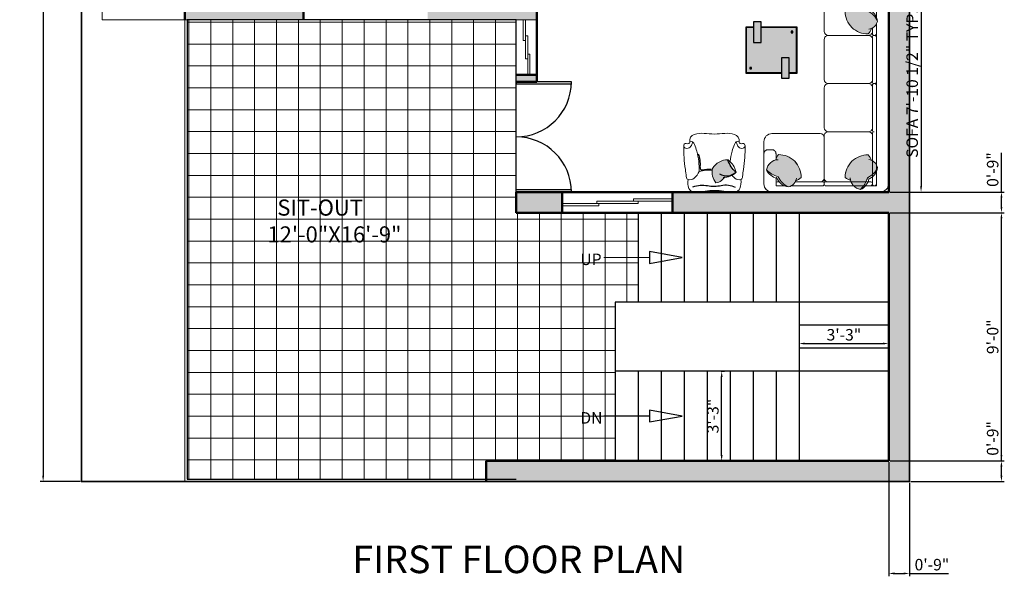
# Model space of a CAD drawing. Units: inches. Extents: x 1734 to 4011, y 1071 to 1891.
# Tile 24 of 27: x 3583 to 4011, y 1071 to 1313. Entities that reach past the tile are written whole.
import ezdxf

# ---------------------------------------------------------------- set-up
doc = ezdxf.new("R2010")
doc.units = ezdxf.units.IN
for name, color, linetype, lineweight in [('A-ANNO-DIMS', 2, 'Continuous', 18), ('A-ANNO-TEXT', 7, 'Continuous', 25), ('A-AREA-IDEN', 3, 'Continuous', 18), ('A-DOOR', 3, 'Continuous', 25), ('A-FLOR-OTLN', 7, 'Continuous', 25), ('A-FLOR-PATT', 252, 'Continuous', 13), ('A-FLOR-STRS', 2, 'Continuous', 25), ('A-FURN', 8, 'Continuous', 18), ('A-FURN-PATT', 252, 'Continuous', 13), ('A-GLAZ', 4, 'Continuous', 18), ('A-WALL', 7, 'Continuous', 50), ('A-WALL-PATT', 8, 'Continuous', 13), ('C-PROP', 1, 'Continuous', 35)]:
    doc.layers.add(name, color=color, linetype=linetype, lineweight=lineweight)
doc.layers.add('IFF-FURN-DETAIL', color=250, linetype='Continuous')
doc.layers.add('MOBIL', color=7, linetype='Continuous')
doc.styles.get("Standard").update_dxf_attribs({"font": 'arial.ttf'})
doc.dimstyles.new('ISO-25', dxfattribs={"dimtxt": 5, "dimasz": 2.5, "dimexe": 1.25, "dimexo": 0.625, "dimtad": 1, "dimdec": 1, "dimlunit": 3, "dimtxsty": 'Standard', "dimcen": 2.5, "dimclrt": 1, "dimadec": 0, "dimazin": 0, "dimtfac": 1, "dimtdec": 1, "dimtmove": 0, "dimatfit": 3, "dimfxl": 1, "dimarcsym": 0})

# ---------------------------------------------------------------- blocks, each defined once
blk = doc.blocks.new('*D59')
at = {"layer": 'A-ANNO-DIMS', "color": 0, "lineweight": -2, "transparency": 16777216}
for p, q in [((3609.2, 1831.82), (3591.89, 1831.82)), ((3593.14, 1829.32), (3593.14, 1114.32)), ((3609.2, 1111.82), (3591.89, 1111.82))]:
    blk.add_line(p, q, dxfattribs=at)
at = {"layer": 'A-ANNO-DIMS', "color": 0, "transparency": 16777216}
for points in [[(3592.73, 1829.32), (3593.56, 1829.32), (3593.14, 1831.82)], [(3592.73, 1114.32), (3593.56, 1114.32), (3593.14, 1111.82)]]:
    blk.add_solid(points, dxfattribs=at)
at = {"layer": 'Defpoints', "color": 0, "transparency": 16777216}
for p in [(3609.83, 1831.82), (3593.14, 1111.82), (3609.83, 1111.82)]:
    blk.add_point(p, dxfattribs=at)
at = {"layer": 'A-ANNO-DIMS', "color": 0, "transparency": 16777216, "insert": (3587.92, 1471.82), "char_height": 5, "attachment_point": 5, "rotation": 90}
blk.add_mtext("{\\H1.8x;60'}", dxfattribs=at)
blk = doc.blocks.new('*D60')
at = {"layer": 'A-ANNO-DIMS', "color": 0, "lineweight": -2, "transparency": 16777216}
for p, q in [((3888.02, 1159.82), (3889.43, 1159.82)), ((3888.18, 1123.32), (3888.18, 1157.32)), ((3888.02, 1120.82), (3889.43, 1120.82))]:
    blk.add_line(p, q, dxfattribs=at)
at = {"layer": 'A-ANNO-DIMS', "color": 0, "transparency": 16777216}
for points in [[(3887.76, 1157.32), (3888.59, 1157.32), (3888.18, 1159.82)], [(3887.76, 1123.32), (3888.59, 1123.32), (3888.18, 1120.82)]]:
    blk.add_solid(points, dxfattribs=at)
at = {"layer": 'Defpoints', "color": 0, "transparency": 16777216}
for p in [(3887.4, 1159.82), (3888.18, 1159.82), (3887.4, 1120.82)]:
    blk.add_point(p, dxfattribs=at)
at = {"layer": 'A-ANNO-DIMS', "color": 0, "transparency": 16777216, "insert": (3885, 1140.32), "char_height": 5, "attachment_point": 5, "rotation": 90}
blk.add_mtext('3\'-3"', dxfattribs=at)
blk = doc.blocks.new('*D61')
at = {"layer": 'A-ANNO-DIMS', "color": 0, "lineweight": -2, "transparency": 16777216}
for p, q in [((3921.83, 1174.19), (3921.83, 1170.62)), ((3960.83, 1174.19), (3960.83, 1170.62)), ((3924.33, 1171.87), (3958.33, 1171.87))]:
    blk.add_line(p, q, dxfattribs=at)
at = {"layer": 'A-ANNO-DIMS', "color": 0, "transparency": 16777216}
for points in [[(3924.33, 1172.28), (3924.33, 1171.45), (3921.83, 1171.87)], [(3958.33, 1172.28), (3958.33, 1171.45), (3960.83, 1171.87)]]:
    blk.add_solid(points, dxfattribs=at)
at = {"layer": 'Defpoints', "color": 0, "transparency": 16777216}
for p in [(3921.83, 1174.82), (3960.83, 1174.82), (3960.83, 1171.87)]:
    blk.add_point(p, dxfattribs=at)
at = {"layer": 'A-ANNO-DIMS', "color": 0, "transparency": 16777216, "insert": (3941.33, 1175.04), "char_height": 5, "attachment_point": 5}
blk.add_mtext('3\'-3"', dxfattribs=at)
blk = doc.blocks.new('Mesa de centro Cantria feeling')
at = {"layer": 'MOBIL', "ltscale": 0.2}
h = blk.add_hatch(color=256, dxfattribs=at)
h.set_gradient(color1=(74, 55, 38), color2=(104, 77, 54), one_color=1, tint=0.31, name='CYLINDER')
h.paths.add_polyline_path([(-0.85, -0.3), (-0.7, -0.3), (-0.7, 0.1), (-0.85, 0.1)])
h = blk.add_hatch(color=256, dxfattribs=at)
h.set_gradient(color1=(221, 221, 223), one_color=1, tint=1)
h.paths.add_polyline_path([(-0.15, -0.6), (-0.15, -0.89), (-0.01, -0.89), (-0.01, -0.01), (-0.7, -0.01), (-0.7, -0.3), (-0.85, -0.3), (-0.85, -0.01), (-0.99, -0.01), (-0.99, -0.89), (-0.3, -0.89), (-0.3, -0.6)])
h.paths.add_polyline_path([(-0.112, -0.112), (-0.112, -0.082), (-0.082, -0.082), (-0.082, -0.112)], flags=16)
h.paths.add_polyline_path([(-0.888, -0.788), (-0.888, -0.818), (-0.918, -0.818), (-0.918, -0.788)], flags=16)
h = blk.add_hatch(color=256, dxfattribs=at)
h.set_gradient(color1=(74, 55, 38), color2=(104, 77, 54), one_color=1, tint=0.31, name='CYLINDER')
h.paths.add_polyline_path([(-0.15, -0.6), (-0.3, -0.6), (-0.3, -1), (-0.15, -1)])
for points in [[(-0.85, 0), (-1, 0), (-1, -0.9), (-0.3, -0.9)], [(-0.15, -0.9), (0, -0.9), (0, 0), (-0.7, 0)], [(-0.85, -0.01), (-0.99, -0.01), (-0.99, -0.89), (-0.3, -0.89)], [(-0.15, -0.89), (-0.01, -0.89), (-0.01, -0.01), (-0.7, -0.01)]]:
    blk.add_lwpolyline(points, dxfattribs=at)
for points in [[(-0.85, -0.3), (-0.7, -0.3), (-0.7, 0.1), (-0.85, 0.1)], [(-0.082, -0.082), (-0.112, -0.082), (-0.112, -0.112), (-0.082, -0.112)], [(-0.15, -0.6), (-0.3, -0.6), (-0.3, -1), (-0.15, -1)], [(-0.918, -0.818), (-0.888, -0.818), (-0.888, -0.788), (-0.918, -0.788)]]:
    blk.add_lwpolyline(points, close=True, dxfattribs=at)
blk = doc.blocks.new("MD D 4'")
for p, q in [((0, 24), (0, 0)), ((1, 24), (1, 0)), ((47, 24), (47, 0)), ((48, 24), (48, 0)), ((0, 0), (1, 0)), ((48, 0), (47, 0))]:
    blk.add_line(p, q)
for centre, start, end in [((0, 0), 0, 90), ((48, 0), 90, 180)]:
    blk.add_arc(centre, 24, start, end)
blk = doc.blocks.new('SOFA 1')
at = {"transparency": 33554687}
h = blk.add_hatch(color=256, dxfattribs=at)
h.dxf.hatch_style = 1
h.paths.add_polyline_path([(3723.52, 1308.63, 0.147724), (3717.76, 1305.24, 0.310469), (3722.42, 1300.4), (3722.42, 1300.25, 0.156703), (3723.62, 1297.8, 0.425821), (3734.69, 1309.08, 0.121928), (3732.05, 1310.63, 0.233216), (3728.6, 1313.59, 0.213835)])
h = blk.add_hatch(color=256, dxfattribs=at)
h.dxf.hatch_style = 1
h.paths.add_polyline_path([(3769.65, 1307.6, 0.084911), (3767.15, 1309.12, 0.046133), (3766.46, 1311.13), (3759.18, 1311.13, 0.039409), (3758.92, 1310.24, 0.165523), (3756.31, 1309.02, 0.42585), (3767.59, 1297.95, 0.121928), (3769.15, 1300.58, 0.027403), (3769.65, 1300.83)])
h.paths.add_polyline_path([(3765.34, 1313.08), (3760.4, 1313.08, 0.097704), (3759.18, 1311.13), (3766.46, 1311.13, 0.04873)])
h.paths.add_polyline_path([(3763.76, 1314.88, 0.16488), (3760.4, 1313.08), (3765.34, 1313.08, 0.051917)])
h.paths.add_polyline_path([(3771.6, 1305.17, 0.090388), (3769.65, 1307.6), (3769.65, 1300.83, 0.136035), (3771.6, 1302.77)])
h = blk.add_hatch(color=256, dxfattribs=at)
h.dxf.hatch_style = 1
h.paths.add_polyline_path([(3769.16, 1235.96, 0.122267), (3767.6, 1238.61, 0.425972), (3756.32, 1227.54, 0.165563), (3758.93, 1226.32, 0.309481), (3763.76, 1221.69, 0.002677), (3763.83, 1221.72, 0.146094), (3767.16, 1227.43, 0.212433), (3772.1, 1232.48, 0.235342)])
h = blk.add_hatch(color=256, dxfattribs=at)
h.dxf.hatch_style = 1
h.paths.add_polyline_path([(3769.16, 1225.36, 0.122267), (3767.6, 1228.01, 0.425972), (3756.32, 1216.94, 0.165563), (3758.93, 1215.72, 0.309481), (3763.76, 1211.09, 0.002677), (3763.83, 1211.12, 0.146094), (3767.16, 1216.83, 0.212433), (3772.1, 1221.88, 0.235342)])
for p, q in [((3720.45, 1316.13), (3773.58, 1316.13)), ((3777.51, 1312.19), (3777.51, 1213.72))]:
    blk.add_line(p, q, dxfattribs=at)
for points in [[(3716.51, 1312.2), (3716.51, 1291.44)], [(3722.42, 1313.08), (3722.42, 1309.23), (3722.42, 1313.08), (3726.57, 1313.08)], [(3729.85, 1313.08), (3745.25, 1313.08)], [(3746.01, 1312.3), (3746.01, 1288.55)], [(3768.11, 1313.08), (3746.78, 1313.08)], [(3771.6, 1313.08), (3767.75, 1313.08), (3771.6, 1313.08), (3771.6, 1308.93)], [(3769.66, 1287.39), (3769.65, 1312.3)], [(3771.6, 1313.08), (3771.61, 1233.74)], [(3723.21, 1311.13), (3723.93, 1311.13)], [(3731.82, 1311.13), (3745.25, 1311.13)], [(3746.01, 1310.97), (3746.01, 1311.36)], [(3746.01, 1288.54), (3746.01, 1308.23)], [(3768.87, 1311.13), (3746.78, 1311.13)], [(3769.65, 1309.43), (3769.65, 1308.71)], [(3722.42, 1300.39), (3722.42, 1297.33)], [(3720.45, 1295.38), (3718.48, 1295.38)], [(3720.45, 1287.5), (3744.09, 1287.5)], [(3746.02, 1284.63), (3746.02, 1264.94)], [(3747.99, 1286.6), (3767.69, 1286.6)], [(3769.66, 1263.75), (3769.66, 1285.81)], [(3769.66, 1277.18), (3769.66, 1263.75)], [(3746.02, 1260.99), (3746.02, 1241.3)], [(3747.99, 1262.97), (3767.69, 1262.97)], [(3769.66, 1240.12), (3769.66, 1262.18)], [(3770.43, 1262.97), (3770.82, 1262.97)], [(3746.02, 1237.36), (3746.02, 1213.74)], [(3747.99, 1239.33), (3767.69, 1239.33)], [(3769.66, 1235.71), (3769.66, 1238.54)], [(3770.43, 1239.33), (3770.82, 1239.33)], [(3771.61, 1223.14), (3771.61, 1230.47)], [(3769.66, 1225.11), (3769.66, 1227.82)], [(3755.86, 1215.72), (3758.92, 1215.72)], [(3767.76, 1215.72), (3771.61, 1215.72), (3771.61, 1219.84), (3771.61, 1215.72)], [(3769.66, 1216.5), (3769.66, 1217.22)], [(3753.91, 1211.77), (3753.91, 1213.74)], [(3749.97, 1209.8), (3773.58, 1209.8)]]:
    blk.add_lwpolyline(points, close=True, dxfattribs=at)
for points in [[(3717.76, 1305.24, -0.147724), (3723.52, 1308.63, -0.213355), (3728.59, 1313.59, 0.213355), (3723.52, 1308.63, 0.147724), (3717.76, 1305.24, -0.249545), (3722.86, 1309.34, 0.249545), (3717.75, 1305.25, 0.356779), (3723.4, 1300.28, -0.356779), (3717.76, 1305.24)], [(3728.58, 1313.6, -0.306333), (3732.42, 1309.31, 0.306333), (3728.58, 1313.6, 0.306674), (3722.72, 1308.89, -0.306674), (3728.58, 1313.6)], [(3763.76, 1314.88, -0.147724), (3767.15, 1309.12, -0.213355), (3772.1, 1304.05, 0.213355), (3767.15, 1309.12, 0.147724), (3763.76, 1314.88, -0.249545), (3767.86, 1309.77, 0.249545), (3763.77, 1314.89, 0.356779), (3758.8, 1309.23, -0.356779), (3763.76, 1314.88)], [(3734.69, 1309.08, -0.425972), (3723.62, 1297.8, -0.165552), (3722.4, 1300.4, 0.165552), (3723.62, 1297.79, 0.425972), (3734.69, 1309.07, 0.121514), (3732.07, 1310.63, -0.121514), (3734.69, 1309.08)], [(3767.6, 1297.95, -0.425972), (3756.31, 1309.01, -0.165552), (3758.92, 1310.24, 0.165552), (3756.31, 1309.02, 0.425972), (3767.59, 1297.95, 0.121514), (3769.14, 1300.57, -0.121514), (3767.6, 1297.95)], [(3772.11, 1304.06, -0.306333), (3767.83, 1300.22, 0.306333), (3772.11, 1304.06, 0.306674), (3767.4, 1309.91, -0.306674), (3772.11, 1304.06)], [(3770.44, 1286.63, -0.414214), (3769.66, 1287.4, 0.414214), (3770.44, 1286.63, 0.414214), (3769.66, 1285.83, -0.414214), (3770.44, 1286.63)], [(3748.01, 1262.99, -0.414214), (3746.05, 1264.95, 0.414214), (3748.01, 1262.97, 0.414213), (3746.05, 1261.01, -0.414213), (3748.01, 1262.99)], [(3770.44, 1262.99, -0.414214), (3769.66, 1263.77, 0.414214), (3770.44, 1262.99, 0.414214), (3769.66, 1262.19, -0.414214), (3770.44, 1262.99)], [(3770.83, 1262.97, -0.414214), (3771.61, 1262.19, 0.414214), (3770.83, 1262.99, 0.414214), (3771.61, 1263.77, -0.414214), (3770.83, 1262.97)], [(3748.01, 1239.35, -0.414214), (3746.05, 1241.31, 0.414214), (3748.01, 1239.33, 0.414213), (3746.05, 1237.37, -0.414213), (3748.01, 1239.35)], [(3767.7, 1239.33, -0.414214), (3769.66, 1237.37, 0.414214), (3767.7, 1239.35, 0.414214), (3769.66, 1241.31, -0.414214), (3767.7, 1239.33)], [(3770.44, 1239.35, -0.414214), (3769.66, 1240.13, 0.414214), (3770.44, 1239.33, 0.414214), (3769.66, 1238.55, -0.414214), (3770.44, 1239.35)], [(3770.83, 1239.33, -0.414214), (3771.61, 1238.55, 0.414214), (3770.83, 1239.35, 0.414214), (3771.61, 1240.13, -0.414214), (3770.83, 1239.33)], [(3756.32, 1227.54, -0.425972), (3767.6, 1238.61, -0.121514), (3769.16, 1235.98, 0.121514), (3767.6, 1238.61, 0.425972), (3756.32, 1227.54, 0.165552), (3758.93, 1226.32, -0.165552), (3756.32, 1227.54)], [(3772.1, 1232.5, -0.306674), (3767.41, 1226.64, 0.306674), (3772.1, 1232.5, 0.306333), (3767.84, 1236.34, -0.306333), (3772.1, 1232.5)], [(3763.78, 1221.67, 0.249545), (3767.87, 1226.78, -0.249545), (3763.76, 1221.69, -0.356779), (3758.81, 1227.32, 0.356779), (3763.77, 1221.68, 0.147724), (3767.16, 1227.43, 0.213355), (3772.11, 1232.51, -0.213355), (3767.16, 1227.43, -0.147724), (3763.78, 1221.67)], [(3756.32, 1216.94, -0.200233), (3759.49, 1224.76, 0.200233), (3756.32, 1216.94, 0.165552), (3758.93, 1215.72, -0.165552), (3756.32, 1216.94)], [(3772.1, 1221.9, -0.306674), (3767.41, 1216.04, 0.306674), (3772.1, 1221.9, -0.213355), (3767.16, 1216.83, -0.147724), (3763.77, 1211.08, 0.147724), (3767.15, 1216.83, 0.213355), (3772.1, 1221.9)], [(3763.76, 1211.09, -0.356779), (3758.81, 1216.72, 0.356779), (3763.76, 1211.09, 0.249545), (3767.87, 1216.18, -0.249545), (3763.76, 1211.09)]]:
    blk.add_lwpolyline(points, format="xyb", dxfattribs=at)
for points in [[(3722.42, 1311.91, 0.414214), (3723.2, 1311.13, -0.414214)], [(3770.43, 1313.08, 0.414214), (3769.65, 1312.3, -0.414214)], [(3771.6, 1312.3, 0.414214), (3770.82, 1313.08, -0.414214)], [(3716.51, 1297.34, 0.414214), (3718.47, 1295.38, -0.414214)], [(3720.44, 1295.38, 0.414214), (3722.4, 1297.34, -0.414214)], [(3716.51, 1291.45, 0.414212), (3720.44, 1287.52, -0.414212)], [(3746.03, 1288.56, 0.414214), (3747.99, 1286.6, 0.414213), (3746.03, 1284.64, -0.414213), (3747.99, 1286.6, -0.414214)], [(3769.66, 1284.64, 0.414214), (3767.7, 1286.6, 0.414214), (3769.66, 1288.56, -0.414214), (3767.7, 1286.6, -0.414214)], [(3769.66, 1261.01, 0.414214), (3767.7, 1262.97, 0.414214), (3769.66, 1264.93, -0.414214), (3767.7, 1262.97, -0.414214)], [(3772.13, 1221.9, 0.306333), (3767.84, 1225.74, -0.306333)], [(3769.16, 1225.36, 0.071861), (3768.39, 1227.01, -0.071861)], [(3755.87, 1215.72, 0.414214), (3753.91, 1213.76, -0.414214)], [(3769.66, 1216.52, 0.414214), (3770.44, 1215.74, -0.414214)], [(3770.83, 1215.74, 0.414214), (3771.61, 1216.52, -0.414214)], [(3746.05, 1213.76, 0.414212), (3749.98, 1209.82, -0.414212)], [(3755.87, 1209.8, -0.414214), (3753.91, 1211.76, 0.414214)]]:
    blk.add_lwpolyline(points, format="xyb", close=True, dxfattribs=at)
for centre, radius, start, end in [((3720.44, 1312.2), 3.93, 90.0002, 179.9998), ((3720.44, 1312.19), 3.94, 89.9158, 179.9154), ((3745.22, 1312.29), 0.789, 0.8425, 90.8425), ((3745.24, 1311.91), 0.777, 270, 0), ((3745.24, 1311.91), 0.777, 270, 0), ((3746.8, 1312.29), 0.789, 89.1575, 179.1575), ((3746.79, 1311.91), 0.777, 180, 270), ((3746.79, 1311.91), 0.777, 180, 270), ((3768.87, 1312.3), 0.777, 360, 90), ((3768.87, 1311.91), 0.777, 270, 0), ((3773.58, 1312.2), 3.93, 0.0002, 89.9998), ((3773.57, 1312.19), 3.94, 359.9158, 89.9154), ((3744.09, 1309.21), 1.92, 358.766, 90.5111), ((3747.93, 1309.21), 1.92, 89.4889, 181.234), ((3744.08, 1289.48), 1.96, 270, 360), ((3744.08, 1289.48), 1.96, 270, 360), ((3773.58, 1213.73), 3.93, 270.0002, 359.9998), ((3773.59, 1213.73), 3.93, 269.9156, 359.9152)]:
    blk.add_arc(centre, radius, start, end, dxfattribs=at)
blk = doc.blocks.new('PILLOW-1')
at = {"color": 0}
blk.add_lwpolyline([(198, -165, -0.232884), (126, -346, -0.184752), (-44, -234, -0.286563), (75, -22, -0.237978), (273, -68, -0.243587), (179, -195, 4.263709)], format="xyb", dxfattribs=at)
at = {"layer": 'IFF-FURN-DETAIL'}
blk.add_lwpolyline([(148, -118, -0.343333), (126, -342, 0.126408), (-40, -233, -5.969376)], format="xyb", dxfattribs=at)
blk = doc.blocks.new('CLNG90')
for points in [[(689, 370, 0.157831), (677, 385, 0.121013), (646, 395, -0.017334), (547, 407, 0.041496), (215, 431, 0.153531), (191, 423, 0.382906), (185, 395, -0.284047), (184, 361, 0.011997), (177, 351, -0.370479), (160, 345, 0.380647), (56, 282, 0.117468), (41, 146, -0.027775), (50, 0, -8.773898)], [(160, 345, 0.22481), (160, 306, 0.055398), (209, 322, 0.180116), (249, 368, 0.194833), (248, 405, 0.242377), (215, 431, 1.52074)], [(160, 345, 0.22481), (160, 306, 0.055398), (209, 322, 0.180116), (249, 368, 0.194833), (248, 405, 0.242377), (215, 431, 1.52074)], [(689, 370, -0.235486), (671, 286, -0.134038), (574, 215, -0.079303), (293, 248, -0.027048), (199, 280, -0.106276), (160, 306, -1.699)], [(689, 370, -0.235486), (671, 286, -0.134038), (574, 215, -0.079303), (293, 248, -0.027048), (199, 280, -0.106276), (160, 306, -1.699)], [(689, 370, -0.146607), (814, 357, -0.305296), (862, 286, -0.042137), (852, 131, 0.040285), (843, 0, 3.952121)], [(574, 215, 0.061244), (556, 29, 3.376255)], [(574, 215, 0.061244), (556, 29, 3.376255)], [(689, -370, -0.157831), (677, -385, -0.121013), (646, -395, 0.017334), (547, -407, -0.041496), (215, -431, -0.153531), (191, -423, -0.382906), (185, -395, 0.284047), (184, -361, -0.011997), (177, -351, 0.370479), (160, -345, -0.380647), (56, -282, -0.117468), (41, -146, 0.027775), (50, 0, 8.773898)], [(689, -370, 0.146607), (814, -357, 0.305296), (862, -286, 0.042137), (852, -131, -0.040285), (843, 0, -3.952121)], [(437, -220, 0.041086), (293, -248, 0.027048), (199, -280, 0.106276), (160, -306, 1.699)], [(437, -220, 0.041086), (293, -248, 0.027048), (199, -280, 0.106276), (160, -306, 1.699)], [(689, -370, 0.235486), (671, -286, 0.060693), (632, -247, 0.001296)], [(689, -370, 0.235486), (671, -286, 0.060693), (632, -247, 0.001296)], [(160, -345, -0.22481), (160, -306, -0.055398), (209, -322, -0.180116), (249, -368, -0.194833), (248, -405, -0.242377), (215, -431, -1.52074)], [(160, -345, -0.22481), (160, -306, -0.055398), (209, -322, -0.180116), (249, -368, -0.194833), (248, -405, -0.242377), (215, -431, -1.52074)]]:
    blk.add_lwpolyline(points, format="xyb")
at = {"layer": 'IFF-FURN-DETAIL'}
for points in [[(791, 301, 0.124986), (774, 96, -0.091334), (771, -95, 0.164688), (797, -292, 1.068868)], [(791, 301, 0.124986), (774, 96, -0.091334), (771, -95, 0.164688), (797, -292, 1.068868)], [(328, 228, 0.109125), (508, 203, -0.16587), (546, 194, -0.314359), (555, 172, 0.072017), (544, 42, 4.351186)], [(328, 228, 0.109125), (508, 203, -0.16587), (546, 194, -0.314359), (555, 172, 0.072017), (544, 42, 4.351186)]]:
    blk.add_lwpolyline(points, format="xyb", dxfattribs=at)
at = {"xscale": 1.016, "yscale": 1.016, "zscale": 1.016}
blk.add_blockref('PILLOW-1', (458, 47), dxfattribs=at)
blk.add_blockref('PILLOW-1', (458, 47), dxfattribs=at)
blk = doc.blocks.new('*D85')
at = {"layer": 'A-ANNO-DIMS', "color": 0, "lineweight": -2, "transparency": 16777216}
for p, q in [((3961.35, 1332.21), (3976.13, 1332.21)), ((3974.88, 1329.71), (3974.88, 1240.32)), ((3961.35, 1237.82), (3976.13, 1237.82))]:
    blk.add_line(p, q, dxfattribs=at)
at = {"layer": 'A-ANNO-DIMS', "color": 0, "transparency": 16777216}
for points in [[(3974.47, 1329.71), (3975.3, 1329.71), (3974.88, 1332.21)], [(3974.47, 1240.32), (3975.3, 1240.32), (3974.88, 1237.82)]]:
    blk.add_solid(points, dxfattribs=at)
at = {"layer": 'Defpoints', "color": 0, "transparency": 16777216}
for p in [(3960.72, 1332.21), (3960.72, 1237.82), (3974.88, 1237.82)]:
    blk.add_point(p, dxfattribs=at)
at = {"layer": 'A-ANNO-DIMS', "color": 1, "transparency": 16777216, "insert": (3971.67, 1285.01), "char_height": 5, "attachment_point": 5, "rotation": 90}
blk.add_mtext('SOFA 7\'-10 1/2" TYP.', dxfattribs=at)
blk = doc.blocks.new('*D131')
at = {"layer": 'A-ANNO-DIMS', "color": 0, "lineweight": -2, "transparency": 16777216}
for p, q in [((4009.83, 1120.82), (4009.83, 1137.86)), ((3961.45, 1120.82), (4011.08, 1120.82)), ((4009.83, 1114.32), (4009.83, 1118.32)), ((3970.45, 1111.82), (4011.08, 1111.82))]:
    blk.add_line(p, q, dxfattribs=at)
at = {"layer": 'A-ANNO-DIMS', "color": 0, "transparency": 16777216}
for points in [[(4009.41, 1118.32), (4010.24, 1118.32), (4009.83, 1120.82)], [(4009.41, 1114.32), (4010.24, 1114.32), (4009.83, 1111.82)]]:
    blk.add_solid(points, dxfattribs=at)
at = {"layer": 'Defpoints', "color": 0, "transparency": 16777216}
for p in [(3960.83, 1120.82), (4009.83, 1120.82), (3969.83, 1111.82)]:
    blk.add_point(p, dxfattribs=at)
at = {"layer": 'A-ANNO-DIMS', "color": 1, "transparency": 16777216, "insert": (4006.65, 1130.59), "char_height": 5, "attachment_point": 5, "rotation": 90}
blk.add_mtext('0\'-9"', dxfattribs=at)
blk = doc.blocks.new('*D132')
at = {"layer": 'A-ANNO-DIMS', "color": 0, "lineweight": -2, "transparency": 16777216}
for p, q in [((3961.45, 1228.82), (4011.08, 1228.82)), ((4009.83, 1123.32), (4009.83, 1226.32)), ((3961.45, 1120.82), (4011.08, 1120.82))]:
    blk.add_line(p, q, dxfattribs=at)
at = {"layer": 'A-ANNO-DIMS', "color": 0, "transparency": 16777216}
for points in [[(4009.41, 1226.32), (4010.24, 1226.32), (4009.83, 1228.82)], [(4009.41, 1123.32), (4010.24, 1123.32), (4009.83, 1120.82)]]:
    blk.add_solid(points, dxfattribs=at)
at = {"layer": 'Defpoints', "color": 0, "transparency": 16777216}
for p in [(3960.83, 1228.82), (4009.83, 1228.82), (3960.83, 1120.82)]:
    blk.add_point(p, dxfattribs=at)
at = {"layer": 'A-ANNO-DIMS', "color": 1, "transparency": 16777216, "insert": (4006.65, 1174.82), "char_height": 5, "attachment_point": 5, "rotation": 90}
blk.add_mtext('9\'-0"', dxfattribs=at)
blk = doc.blocks.new('*D133')
at = {"layer": 'A-ANNO-DIMS', "color": 0, "lineweight": -2, "transparency": 16777216}
for p, q in [((4009.83, 1237.82), (4009.83, 1254.86)), ((3961.45, 1237.82), (4011.08, 1237.82)), ((4009.83, 1231.32), (4009.83, 1235.32)), ((3961.45, 1228.82), (4011.08, 1228.82))]:
    blk.add_line(p, q, dxfattribs=at)
at = {"layer": 'A-ANNO-DIMS', "color": 0, "transparency": 16777216}
for points in [[(4009.41, 1235.32), (4010.24, 1235.32), (4009.83, 1237.82)], [(4009.41, 1231.32), (4010.24, 1231.32), (4009.83, 1228.82)]]:
    blk.add_solid(points, dxfattribs=at)
at = {"layer": 'Defpoints', "color": 0, "transparency": 16777216}
for p in [(3960.83, 1237.82), (4009.83, 1237.82), (3960.83, 1228.82)]:
    blk.add_point(p, dxfattribs=at)
at = {"layer": 'A-ANNO-DIMS', "color": 1, "transparency": 16777216, "insert": (4006.65, 1247.59), "char_height": 5, "attachment_point": 5, "rotation": 90}
blk.add_mtext('0\'-9"', dxfattribs=at)
blk = doc.blocks.new('*D134')
at = {"layer": 'A-ANNO-DIMS', "color": 0, "lineweight": -2, "transparency": 16777216}
for p, q in [((3960.83, 1120.19), (3960.83, 1070.57)), ((3969.83, 1111.19), (3969.83, 1070.57)), ((3963.33, 1071.82), (3967.33, 1071.82)), ((3969.83, 1071.82), (3986.87, 1071.82))]:
    blk.add_line(p, q, dxfattribs=at)
at = {"layer": 'A-ANNO-DIMS', "color": 0, "transparency": 16777216}
for points in [[(3963.33, 1072.24), (3963.33, 1071.4), (3960.83, 1071.82)], [(3967.33, 1072.24), (3967.33, 1071.4), (3969.83, 1071.82)]]:
    blk.add_solid(points, dxfattribs=at)
at = {"layer": 'Defpoints', "color": 0, "transparency": 16777216}
for p in [(3960.83, 1120.82), (3969.83, 1111.82), (3969.83, 1071.82)]:
    blk.add_point(p, dxfattribs=at)
at = {"layer": 'A-ANNO-DIMS', "color": 1, "transparency": 16777216, "insert": (3979.6, 1075), "char_height": 5, "attachment_point": 5}
blk.add_mtext('0\'-9"', dxfattribs=at)

msp = doc.modelspace()

# ---------------------------------------------------------------- hatches: boundary and pattern name
at = {"layer": 'A-FLOR-PATT'}
h = msp.add_hatch(dxfattribs=at)
h.set_pattern_fill('ANSI37', color=256, scale=3, angle=45)
h.set_pattern_definition([(90, (598.983, -12.241), (-9.525, 0), []), (180, (598.983, -12.241), (-9e-16, -9.525), [])])
h.paths.add_polyline_path([(3798.83, 1228.82), (3798.83, 1312.82), (3655.83, 1312.82), (3655.83, 1112.82), (3785.83, 1112.82), (3785.83, 1120.82), (3841.83, 1120.82), (3841.83, 1189.82), (3851.83, 1189.82), (3851.83, 1228.82)])
h.paths.add_polyline_path([(3824.93, 1134.29), (3837.52, 1134.29), (3837.52, 1144.59), (3824.93, 1144.59)], flags=24)
h.paths.add_polyline_path([(3824.92, 1203.29), (3837.13, 1203.29), (3837.13, 1213.59), (3824.92, 1213.59)], flags=24)
h.paths.add_polyline_path([(3687.88, 1211.9), (3747.72, 1211.9), (3747.72, 1238.02), (3687.88, 1238.02)], flags=24)
at = {"layer": 'A-FURN-PATT'}
h = msp.add_hatch(dxfattribs=at)
h.set_pattern_fill('ANSI32', color=256)
h.set_pattern_definition([(45, (598.983, -12.241), (-6.735192, 6.735192), []), (45, (603.473, -12.241), (-6.735192, 6.735192), [])])
h.paths.add_polyline_path([(3723.83, 1453.82), (3663.83, 1453.82), (3663.83, 1435.82), (3723.83, 1435.82)])
h.paths.add_polyline_path([(3667.71, 1440.04), (3717.17, 1440.04), (3717.17, 1450.34), (3667.71, 1450.34)], flags=24)
h.paths.add_polyline_path([(3882.46, 1633.93), (3882.46, 1688.64), (3856.34, 1688.64), (3856.34, 1633.93)], flags=9)
h.paths.add_polyline_path([(3912.44, 1633.93), (3912.44, 1688.64), (3886.32, 1688.64), (3886.32, 1633.93)], flags=9)
h.paths.add_polyline_path([(3849.42, 1795.58), (3903.83, 1795.58), (3903.83, 1821.7), (3849.42, 1821.7)], flags=9)
h.paths.add_polyline_path([(3821.75, 1770.76), (3864.43, 1770.76), (3864.43, 1779), (3821.75, 1779)], flags=9)
h.paths.add_polyline_path([(3824.93, 1134.29), (3837.52, 1134.29), (3837.52, 1144.59), (3824.93, 1144.59)], flags=9)
h.paths.add_polyline_path([(3824.92, 1203.29), (3837.13, 1203.29), (3837.13, 1213.59), (3824.92, 1213.59)], flags=9)
h.paths.add_polyline_path([(3649.53, 1633.93), (3649.53, 1688.64), (3623.41, 1688.64), (3623.41, 1633.93)], flags=9)
h.paths.add_polyline_path([(3861.96, 1555.4), (3916.37, 1555.4), (3916.37, 1581.52), (3861.96, 1581.52)], flags=9)
h.paths.add_polyline_path([(3920.06, 1601.91), (3940.42, 1601.91), (3940.42, 1612.21), (3920.06, 1612.21)], flags=9)
h.paths.add_polyline_path([(3879.75, 1638.04), (3929.21, 1638.04), (3929.21, 1648.34), (3879.75, 1648.34)], flags=9)
h.paths.add_polyline_path([(3861.7, 1695.43), (3921.55, 1695.43), (3921.55, 1721.55), (3861.7, 1721.55)], flags=9)
h.paths.add_polyline_path([(3738.69, 1778.27), (3787.65, 1778.27), (3787.65, 1804.39), (3738.69, 1804.39)], flags=9)
h.paths.add_polyline_path([(3649.33, 1778.26), (3698.3, 1778.26), (3698.3, 1804.38), (3649.33, 1804.38)], flags=9)
h.paths.add_polyline_path([(3687.88, 1211.9), (3747.72, 1211.9), (3747.72, 1238.02), (3687.88, 1238.02)], flags=9)
h.paths.add_polyline_path([(3782.95, 1496.7), (3837.36, 1496.7), (3837.36, 1522.82), (3782.95, 1522.82)], flags=9)
h.paths.add_polyline_path([(3862.83, 1344.86), (3931.88, 1344.86), (3931.88, 1370.98), (3862.83, 1370.98)], flags=9)
h.paths.add_polyline_path([(3887.8, 1472.31), (3942.21, 1472.31), (3942.21, 1498.43), (3887.8, 1498.43)], flags=9)
h.paths.add_polyline_path([(3707.14, 1647.71), (3772.42, 1647.71), (3772.42, 1673.83), (3707.14, 1673.83)], flags=9)
h = msp.add_hatch(color=256, dxfattribs=at)
h.dxf.hatch_style = 1
h.paths.add_polyline_path([(3884.26, 1248.05, 0.237978), (3885.72, 1241.82, 0.250405), (3889.78, 1244.88, 0.218011), (3894.34, 1246.42, -0.129718), (3890.84, 1251.81, 0.283254)])
at = {"layer": 'A-WALL-PATT'}
h = msp.add_hatch(color=256, dxfattribs=at)
h.dxf.hatch_style = 1
h.paths.add_polyline_path([(3969.83, 1831.82), (3618.83, 1831.82), (3618.83, 1745.82), (3627.39, 1745.82), (3627.39, 1750.82), (3623.83, 1750.82), (3623.83, 1822.82), (3710.83, 1822.82), (3710.83, 1780.82), (3715.83, 1780.82), (3715.83, 1822.82), (3802.83, 1822.82), (3802.83, 1750.82), (3750.83, 1750.82), (3750.83, 1745.82), (3802.83, 1745.82), (3802.83, 1604.82), (3807.83, 1604.82), (3807.83, 1628.82), (3811.83, 1628.82), (3811.83, 1633.82), (3807.83, 1633.82), (3807.83, 1777.82), (3813.86, 1777.82), (3813.86, 1786.82), (3807.83, 1786.82), (3807.83, 1826.82), (3960.83, 1826.82), (3960.83, 1786.82), (3942.83, 1786.82), (3942.83, 1777.82), (3960.83, 1777.82), (3960.83, 1633.82), (3847.83, 1633.82), (3847.83, 1628.82), (3960.83, 1628.82), (3960.83, 1588.82), (3912.83, 1588.82), (3912.83, 1585.82), (3960.83, 1585.82), (3960.83, 1517.82), (3946.33, 1517.82), (3946.33, 1512.82), (3960.83, 1512.82), (3960.83, 1458.82), (3940.33, 1458.82), (3940.33, 1453.82), (3969.83, 1453.82)])
h.paths.add_polyline_path([(3969.83, 1453.82), (3960.83, 1453.82), (3960.83, 1237.82), (3866.83, 1237.82), (3866.83, 1228.82), (3960.83, 1228.82), (3960.83, 1120.82), (3785.83, 1120.82), (3785.83, 1111.82), (3969.83, 1111.82)])
h = msp.add_hatch(color=256, dxfattribs=at)
h.dxf.hatch_style = 1
h.paths.add_polyline_path([(3663.83, 1530.82), (3654.83, 1530.82), (3654.83, 1351.82), (3663.83, 1351.82), (3663.83, 1453.82), (3757.83, 1453.82), (3757.83, 1458.82), (3728.83, 1458.82), (3728.83, 1470.82), (3723.83, 1470.82), (3723.83, 1458.82), (3663.83, 1458.82)])
h.paths.add_polyline_path([(3706.33, 1321.82), (3654.83, 1321.82), (3654.83, 1312.82), (3706.33, 1312.82)])
h.paths.add_polyline_path([(3807.83, 1453.82), (3812.83, 1453.82), (3812.83, 1458.82), (3793.83, 1458.82), (3793.83, 1453.82), (3802.83, 1453.82), (3802.83, 1321.82), (3760.33, 1321.82), (3760.33, 1312.82), (3807.83, 1312.82)])
h.paths.add_polyline_path([(3807.83, 1288.82), (3798.83, 1288.82), (3798.83, 1285.82), (3807.83, 1285.82)])
h.paths.add_polyline_path([(3807.83, 1568.82), (3802.83, 1568.82), (3802.83, 1564.82), (3659.83, 1564.82), (3659.83, 1569.82), (3654.83, 1569.82), (3654.83, 1554.82), (3663.83, 1554.82), (3663.83, 1559.82), (3723.83, 1559.82), (3723.83, 1500.82), (3728.83, 1500.82), (3728.83, 1559.82), (3807.83, 1559.82)])
h.paths.add_polyline_path([(3659.83, 1623.83), (3654.83, 1623.83), (3654.83, 1599.82), (3659.83, 1599.82)])
h.paths.add_polyline_path([(3720.83, 1750.82), (3651.39, 1750.82), (3651.39, 1745.82), (3654.83, 1745.82), (3654.83, 1671.83), (3659.83, 1671.83), (3659.83, 1745.82), (3720.83, 1745.82)])
h.paths.add_polyline_path([(3818.83, 1237.82), (3798.83, 1237.82), (3798.83, 1228.82), (3818.83, 1228.82)])

# ---------------------------------------------------------------- linework, layer by layer
at = {"layer": 'A-FLOR-OTLN'}
msp.add_lwpolyline([(3798.83, 1228.82), (3798.83, 1312.82), (3655.83, 1312.82), (3655.83, 1112.82), (3798.83, 1112.82)], dxfattribs=at)
at = {"layer": 'A-FLOR-STRS'}
for p, q in [((3851.83, 1228.82), (3851.83, 1189.82)), ((3861.83, 1228.82), (3861.83, 1189.82)), ((3871.83, 1228.82), (3871.83, 1189.82)), ((3881.83, 1228.82), (3881.83, 1189.82)), ((3891.83, 1228.82), (3891.83, 1189.82)), ((3901.83, 1228.82), (3901.83, 1189.82)), ((3911.83, 1228.82), (3911.83, 1189.82)), ((3921.83, 1228.82), (3921.83, 1120.82)), ((3960.83, 1189.82), (3841.83, 1189.82)), ((3841.83, 1189.82), (3841.83, 1120.82)), ((3960.83, 1179.82), (3921.83, 1179.82)), ((3960.83, 1169.82), (3921.83, 1169.82)), ((3960.83, 1159.82), (3841.83, 1159.82)), ((3851.83, 1159.82), (3851.83, 1120.82)), ((3861.83, 1159.82), (3861.83, 1120.82)), ((3871.83, 1159.82), (3871.83, 1120.82)), ((3881.83, 1159.82), (3881.83, 1120.82)), ((3891.83, 1159.82), (3891.83, 1120.82)), ((3901.83, 1159.82), (3901.83, 1120.82)), ((3911.83, 1159.82), (3911.83, 1120.82)), ((3856.83, 1140.32), (3836.91, 1140.32))]:
    msp.add_line(p, q, dxfattribs=at)
for points in [[(3870.98, 1209.32), (3856.83, 1211.87), (3856.83, 1206.77)], [(3870.98, 1140.32), (3856.83, 1142.87), (3856.83, 1137.77)]]:
    msp.add_lwpolyline(points, close=True, dxfattribs=at)
at = {"layer": 'A-FURN'}
for p, q in [((3654.83, 1111.82), (3654.83, 1569.82)), ((3618.83, 1312.82), (3618.83, 1458.82)), ((3618.83, 1312.82), (3807.83, 1312.82)), ((3655.83, 1112.82), (3655.83, 1312.82)), ((3798.83, 1312.82), (3798.83, 1285.82)), ((3856.83, 1209.32), (3836.91, 1209.32)), ((3655.83, 1112.82), (3785.83, 1112.82))]:
    msp.add_line(p, q, dxfattribs=at)
at = {"layer": 'A-GLAZ'}
for p, q in [((3801.83, 1303.82), (3801.83, 1312.82)), ((3802.83, 1295.82), (3802.83, 1312.82)), ((3803.83, 1305.82), (3802.83, 1305.82)), ((3803.83, 1288.82), (3803.83, 1305.82)), ((3802.83, 1303.82), (3801.83, 1303.82)), ((3804.83, 1297.82), (3803.83, 1297.82)), ((3804.83, 1288.82), (3804.83, 1297.82)), ((3803.83, 1295.82), (3802.83, 1295.82)), ((3833.83, 1233.82), (3866.83, 1233.82)), ((3833.83, 1232.82), (3833.83, 1233.82)), ((3849.83, 1234.82), (3866.83, 1234.82)), ((3849.83, 1233.82), (3849.83, 1234.82)), ((3851.83, 1232.82), (3851.83, 1233.82)), ((3818.83, 1232.82), (3851.83, 1232.82)), ((3818.83, 1231.82), (3834.83, 1231.82)), ((3834.83, 1231.82), (3834.83, 1232.82))]:
    msp.add_line(p, q, dxfattribs=at)
at = {"layer": 'A-WALL'}
for p, q in [((3807.83, 1285.82), (3807.83, 1453.82)), ((3960.83, 1453.82), (3960.83, 1237.82)), ((3654.83, 1312.82), (3654.83, 1321.82)), ((3706.33, 1321.82), (3706.33, 1312.82)), ((3807.83, 1288.82), (3798.83, 1288.82)), ((3807.83, 1285.82), (3798.83, 1285.82)), ((3798.83, 1237.82), (3798.83, 1228.82)), ((3960.83, 1237.82), (3798.83, 1237.82)), ((3818.83, 1237.82), (3818.83, 1228.82)), ((3866.83, 1237.82), (3866.83, 1228.82)), ((3960.83, 1228.82), (3798.83, 1228.82)), ((3960.83, 1228.82), (3960.83, 1120.82)), ((3785.83, 1120.82), (3785.83, 1111.82)), ((3960.83, 1120.82), (3785.83, 1120.82))]:
    msp.add_line(p, q, dxfattribs=at)
at = {"layer": 'C-PROP'}
msp.add_lwpolyline([(3785.83, 1111.82), (3609.83, 1111.82), (3609.83, 1831.82), (3969.83, 1831.82), (3969.83, 1111.82), (3785.83, 1111.82)], dxfattribs=at)

# ---------------------------------------------------------------- block references
at = {"layer": 'A-DOOR', "rotation": 270}
msp.add_blockref("MD D 4'", (3798.83, 1285.82), dxfattribs=at)
at = {"layer": 'A-FURN'}
for name, p, xscale, yscale, zscale, rotation in [('SOFA 1', (607.6, 2406.09), -0.887653230693335, 0.887653230693335, 0.887653230693335, 180), ('CLNG90', (3885.03, 1264.61), -0.031001591544, 0.031001591544, 0.031001591544, 90)]:
    msp.add_blockref(name, p, dxfattribs=dict(at, xscale=xscale, yscale=yscale, zscale=zscale, rotation=rotation))
at = {"layer": 'A-FURN', "xscale": 22.3138190187957, "yscale": 22.3138190187957, "zscale": 22.3138190187957}
msp.add_blockref('Mesa de centro Cantria feeling', (3920.94, 1309.63), dxfattribs=at)

# ---------------------------------------------------------------- texts
at = {"layer": 'A-ANNO-TEXT', "attachment_point": 1}
for s, width, insert, char_height in [('UP', 10.7355, (3826.72, 1211.02), 5), ('DN', 10.7355, (3826.72, 1142.02), 5), ('FIRST FLOOR PLAN', 228.5661, (3727.58, 1083.95), 12)]:
    msp.add_mtext_dynamic_manual_height_columns(s, width=width, gutter_width=12.5, heights=[0], dxfattribs=dict(at, insert=insert, char_height=char_height))
at = {"layer": 'A-AREA-IDEN', "insert": (3690.7, 1234.54), "char_height": 7, "attachment_point": 1}
msp.add_mtext_dynamic_manual_height_columns('  SIT-OUT\\P12\'-0"X16\'-9"', width=86.9528, gutter_width=12.5, heights=[0], dxfattribs=at)

# ---------------------------------------------------------------- dimensions: what is measured, and where the dimension line sits
at = {"layer": 'A-ANNO-DIMS'}
for base, p1, p2, angle, text, override, picture, middle in [((3593.14, 1111.82), (3609.83, 1831.82), (3609.83, 1111.82), 90, '{\\H1.8x;<>}', {"dimclrd": 0, "dimclre": 0, "dimclrt": 0}, '*D59', (3587.92, 1471.82)), ((3974.88, 1237.82), (3960.72, 1332.21), (3960.72, 1237.82), 270, 'SOFA <> TYP.', {"dimdec": 1, "dimrnd": 0, "dimzin": 1, "dimlunit": 4, "dimfrac": 2}, '*D85', (3971.67, 1285.01))]:
    dim = msp.add_linear_dim(base=base, p1=p1, p2=p2, angle=angle, text=text, dimstyle='ISO-25', override=override, dxfattribs=at)
    dim.commit()
    dim.dimension.update_dxf_attribs({"geometry": picture, "text_midpoint": middle})
for base, p1, p2, override, picture, middle in [((4009.83, 1237.82), (3960.83, 1228.82), (3960.83, 1237.82), {"dimdec": 1, "dimlfac": 1, "dimrnd": 0, "dimzin": 1, "dimdsep": 46, "dimlunit": 4, "dimfrac": 2}, '*D133', (4006.65, 1247.59)), ((4009.83, 1228.82), (3960.83, 1120.82), (3960.83, 1228.82), {"dimdec": 1, "dimlfac": 1, "dimrnd": 0, "dimzin": 1, "dimdsep": 46, "dimlunit": 4, "dimfrac": 2}, '*D132', (4006.65, 1174.82)), ((3888.18, 1159.82), (3887.4, 1120.82), (3887.4, 1159.82), {"dimclrd": 0, "dimclre": 0, "dimclrt": 0}, '*D60', (3885, 1140.32)), ((4009.83, 1120.82), (3969.83, 1111.82), (3960.83, 1120.82), {"dimdec": 1, "dimlfac": 1, "dimrnd": 0, "dimzin": 1, "dimdsep": 46, "dimlunit": 4, "dimfrac": 2}, '*D131', (4006.65, 1130.59))]:
    dim = msp.add_linear_dim(base=base, p1=p1, p2=p2, angle=90, dimstyle='ISO-25', override=override, dxfattribs=at)
    dim.commit()
    dim.dimension.update_dxf_attribs({"geometry": picture, "text_midpoint": middle})
for base, p1, p2, override, picture, middle in [((3960.83, 1171.87), (3921.83, 1174.82), (3960.83, 1174.82), {"dimclrd": 0, "dimclre": 0, "dimclrt": 0}, '*D61', (3941.33, 1175.04)), ((3969.83, 1071.82), (3960.83, 1120.82), (3969.83, 1111.82), {"dimdec": 1, "dimlfac": 1, "dimrnd": 0, "dimzin": 1, "dimdsep": 46, "dimlunit": 4, "dimfrac": 2}, '*D134', (3979.6, 1075))]:
    dim = msp.add_linear_dim(base=base, p1=p1, p2=p2, dimstyle='ISO-25', override=override, dxfattribs=at)
    dim.commit()
    dim.dimension.update_dxf_attribs({"geometry": picture, "text_midpoint": middle})

doc.saveas('drawing.dxf')
